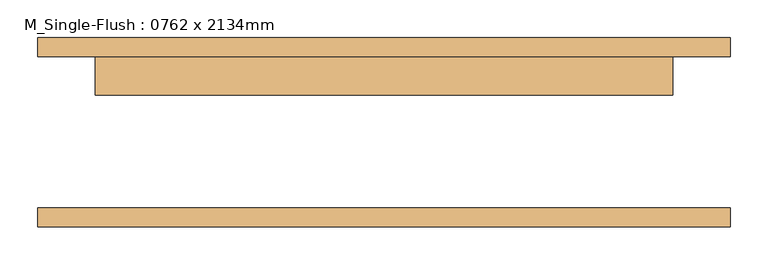
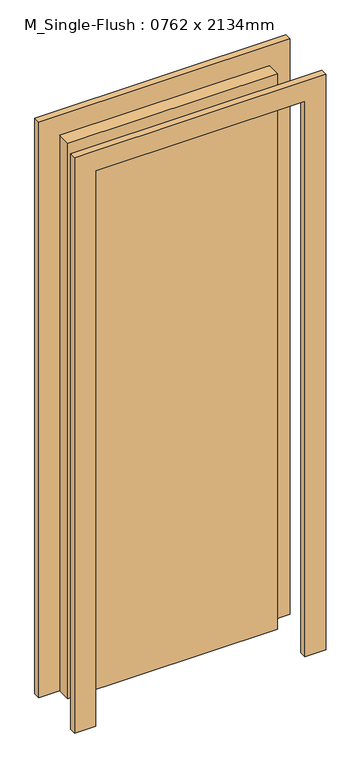
"""IFC4 building model written with IfcOpenShell, lengths in millimetres: door geometry, M_Single-Flush : 0762 x 2134mm."""

from ifc_helpers import new_model, si_unit, frame, origin, origin_with_axes, place, context, project, spatial, polyline, outline, extrude, source, transform, mapped, element, save


def m_single_flush_0762_x_2134mm_85379237(model_context):
    return source(origin(), model_context, "Body", "SweptSolid", [
        extrude(outline(polyline([(2210.0, -457.0), (0.0, -457.0), (0.0, -381.0), (2134.0, -381.0), (2134.0, 381.0), (0.0, 381.0), (0.0, 457.0), (2210.0, 457.0), (2210.0, -457.0)])), frame((0.0, 100.0, 0.0), z_axis=(0.0, 1.0, 0.0), x_axis=(0.0, 0.0, 1.0)), (0.0, 0.0, 1.0), 25.0),
        extrude(outline(polyline([(2210.0, 457.0), (2210.0, -457.0), (0.0, -457.0), (0.0, -381.0), (2134.0, -381.0), (2134.0, 381.0), (0.0, 381.0), (0.0, 457.0), (2210.0, 457.0)])), frame((0.0, -125.0, 0.0), z_axis=(0.0, 1.0, 0.0), x_axis=(0.0, 0.0, 1.0)), (0.0, 0.0, 1.0), 25.0),
        extrude(outline(polyline([(381.0, 49.0), (-381.0, 49.0), (-381.0, 100.0), (381.0, 100.0), (381.0, 49.0)])), origin_with_axes(), (0.0, 0.0, 1.0), 2134.0),
    ])


if __name__ == "__main__":
    model = new_model("IFC4")
    model_context = context("Model", 3, world=origin())
    ifc_project = project(units=[si_unit("LENGTHUNIT", "METRE", prefix="MILLI")], contexts=[model_context])
    site = spatial("IfcSite", under=ifc_project)
    building = spatial("IfcBuilding", under=site)
    placement = place(None, origin())
    m_single_flush_0762_x_2134mm_shape = m_single_flush_0762_x_2134mm_85379237(model_context)
    element("IfcDoor", 1, ObjectType="M_Single-Flush : 0762 x 2134mm", at=placement, inside=building, context=model_context, shape_type="MappedRepresentation", body=[
        mapped(m_single_flush_0762_x_2134mm_shape, transform((0.0, 0.0, 0.0), x_axis=(1.0, 0.0, 0.0), y_axis=(0.0, 1.0, 0.0), z_axis=(0.0, 0.0, 1.0))),
    ])
    save(model, "model.ifc")

# Revit data of these elements
# Type "M_Single-Flush : 0762 x 2134mm"
#   Type Mark = "18"
#   Thickness = 0' - 2.00787"
#   Height = 7' - 0.01575"
#   Trim Projection Ext = 0' - 0.98425"
#   Trim Projection Int = 0' - 0.98425"
#   Trim Width = 0' - 2.99213"
#   Width = 2' - 6"
#   Door Material = Door - Panel
#   Frame Material = Door - Frame
#   Function = (empty or 0)
#   Wall Closure = (empty or 0)
# Element 1 (IfcDoor, "M_Single-Flush : 0762 x 2134mm")
#   Materials on its faces: "Door - Frame", "Door - Panel"
# Materials
#   "Door - Panel": class "Wood", colour RGB 114 82 51, transparency 0
#   "Door - Frame": colour RGB 153 76 43, transparency 0
